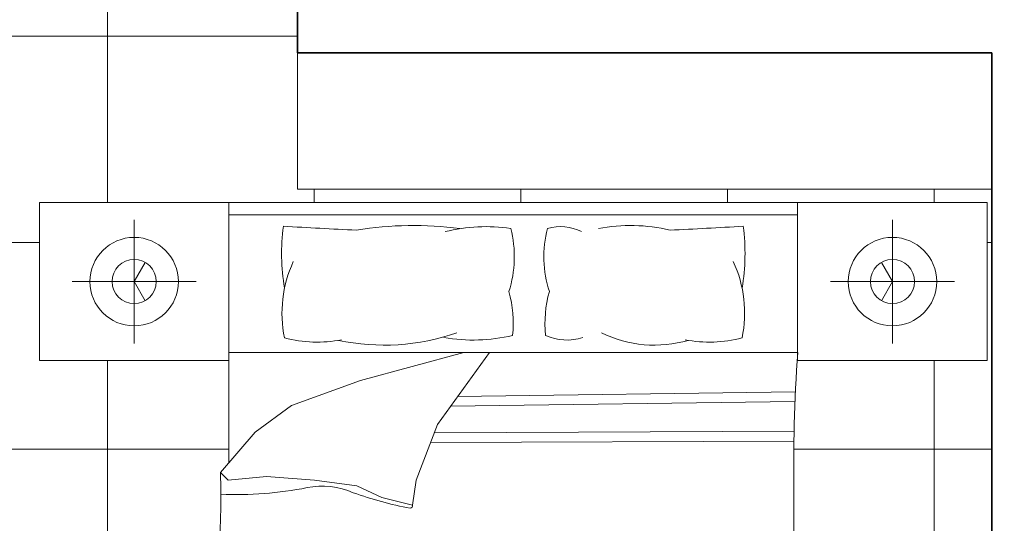
# Model space of a CAD drawing. Units: inches. Extents: x 351 to 1738, y -265 to 286.
# Tile 25 of 38: x 1127 to 1246, y 102 to 163. Entities that reach past the tile are written whole.
import ezdxf

# ---------------------------------------------------------------- set-up
doc = ezdxf.new("R2010")
doc.units = ezdxf.units.IN
doc.header["$MEASUREMENT"] = 0
for name, color, linetype, lineweight in [('A-FLOR-CASE', 9, 'Continuous', 18), ('A-FLOR-PATT', 9, 'Continuous', 9), ('A-FURN', 18, 'Continuous', 13), ('A-WALL', 7, 'Continuous', 35)]:
    doc.layers.add(name, color=color, linetype=linetype, lineweight=lineweight)

msp = doc.modelspace()

# ---------------------------------------------------------------- hatches: boundary and pattern name
at = {"layer": 'A-FLOR-PATT', "transparency": 33554559}
h = msp.add_hatch(dxfattribs=at)
h.set_pattern_fill('ANSI37', color=256, scale=200, angle=135)
h.set_pattern_definition([(180, (1112.704, -164.037), (-2e-15, -25), []), (270, (1112.704, -164.037), (25, -5e-15), [])])
h.paths.add_polyline_path([(1380.064, 73.463), (1380.132, 148.463), (1338.064, 148.463), (1290.704, 148.463), (1290.704, 88.463), (1248.704, 88.463), (1248.704, -2.009), (1244.704, -2.009), (1244.704, 142.457), (1160.704, 142.457), (1160.704, 158.963), (1160.704, 170.137), (1160.704, 206.137), (1160.704, 228.963), (1112.704, 228.963), (1112.704, 209.963), (1112.704, 168.963), (1124.704, 168.963), (1124.704, 162.963), (1112.704, 162.963), (1112.704, 64.463), (1112.704, 60.463), (1112.704, 0.463), (1112.704, -48.026), (1146.804, -47.981), (1146.804, -35.691), (1207.804, -35.691), (1207.804, -47.902), (1236.542, -47.864), (1236.544, -50.009), (1248.5, -50.009), (1248.506, -102.915), (1248.512, -150.915), (1248.514, -164.037), (1248.549, -164.037), (1273.017, -164.037), (1273.017, -128.799), (1355.24, -128.799), (1355.24, -164.037), (1384.204, -164.037), (1384.204, -57.037), (1380.064, -57.037), (1380.064, -48.037), (1392.064, -48.037), (1392.064, -53.037), (1406.549, -53.037), (1406.549, -57.037), (1401.204, -57.037), (1401.204, -147.037), (1468.204, -147.037), (1468.204, -138.5), (1472.204, -138.5), (1472.204, -102.5), (1468.204, -102.5), (1468.204, -57.037), (1442.549, -57.037), (1442.549, -53.037), (1463.049, -53.037), (1463.049, -40.747), (1524.049, -40.747), (1524.049, -48.037), (1536.064, -48.037), (1536.064, -53.037), (1557.704, -53.037), (1557.704, 204.963), (1384.204, 204.963), (1384.204, 73.463), (1392.064, 73.463), (1392.064, 64.463), (1384.204, 64.463), (1384.204, -3.5), (1380.204, -3.537), (1380.204, 64.463), (1380.064, 64.463)])
h.paths.add_polyline_path([(1510.714, 86.458, -0.1039845), (1511.661, 85.595, 0.4704384), (1510.158, 87.614, 0.0961001)], flags=16)
h.paths.add_polyline_path([(1510.443, 100.266, 0.009798), (1504.693, 100.48, 0.0287898), (1504.6, 99.767, -0.1653311), (1505.519, 96.135, -0.1436014)], flags=16)
h.paths.add_polyline_path([(1487.201, 85.595, -0.1039845), (1488.148, 86.458, 0.0961001), (1488.704, 87.614, 0.4704384)], flags=0)
h.paths.add_polyline_path([(1495.052, 100.43), (1494.178, 100.43, -0.0264629), (1494.262, 99.774, -0.1442193)], flags=16)
h.paths.add_polyline_path([(1444.485, 86.458, -0.1039845), (1445.433, 85.595, 0.4704384), (1443.93, 87.614, 0.0961001)], flags=16)
h.paths.add_polyline_path([(1420.972, 85.595, -0.1039845), (1421.92, 86.458, 0.0961001), (1422.475, 87.614, 0.4704384)], flags=16)
h.paths.add_polyline_path([(1428.632, 100.335, 0.0010541), (1427.971, 100.309, -0.0215241), (1428.033, 99.774, -0.1143008)], flags=16)
h.paths.add_polyline_path([(1419.906, 143.708, 0.0249793), (1420.222, 157.526), (1421.573, 159.101), (1421.573, 175.369), (1391.393, 175.369), (1391.393, 200.519), (1542.294, 200.519), (1542.294, 175.369), (1512.028, 175.369, 0.0198653), (1511.521, 153.838, 0.0251335), (1512.758, 118.323, 0.0205529), (1512.942, 115.253), (1419.834, 115.253, -0.0004142), (1419.843, 124.798), (1413.059, 124.798), (1413.059, 84.437, -0.0618528), (1415.831, 80.45, -0.0930773), (1420.972, 85.595, -0.2675367), (1422.371, 84.732, 0.0851103), (1424.052, 84.616, -0.8853927), (1424.033, 84.851, -1.1258145), (1424.073, 84.366, -0.0879871), (1422.371, 84.732, -0.2675367), (1422.326, 83.089, -0.3705421), (1420.972, 85.595, 0.0930773), (1415.831, 80.45, -0.0874142), (1417.914, 73.937), (1418.941, 73.937, 0.0272504), (1418.913, 76.906, -0.1157032), (1421.051, 73.937), (1445.354, 73.937, -0.1157032), (1447.492, 76.906, 0.0272504), (1447.464, 73.937), (1448.491, 73.937, -0.0874142), (1450.574, 80.45, 0.0930773), (1445.433, 85.595, -0.3705421), (1444.079, 83.089, -0.2675367), (1444.034, 84.732, -0.0879871), (1442.332, 84.366, -1.1258145), (1442.372, 84.851, -2.0327363), (1442.364, 84.368, 0.0863779), (1444.034, 84.732, -0.2675367), (1445.433, 85.595, -0.0930773), (1450.574, 80.45, -0.2577317), (1466.483, 90.927, -0.4786702), (1468.832, 91.907, -0.4786702), (1471.18, 90.927, -0.26264), (1483.053, 81.78, -0.0718662), (1487.201, 85.595, -0.2675367), (1488.6, 84.732, 0.0851103), (1490.28, 84.616, -0.8853927), (1490.262, 84.851, -1.1258145), (1490.301, 84.366, -0.0879871), (1488.6, 84.732, -0.2675367), (1488.554, 83.089, -0.3705421), (1487.201, 85.595, 0.0718662), (1483.053, 81.78, -0.1320648), (1484.143, 73.937), (1485.169, 73.937, 0.0272504), (1485.142, 76.906, -0.1157032), (1487.28, 73.937), (1511.582, 73.937, -0.1157032), (1513.72, 76.906, 0.0272504), (1513.693, 73.937), (1514.719, 73.937, -0.0874142), (1516.802, 80.45, 0.0930773), (1511.661, 85.595, -0.3705421), (1510.308, 83.089, -0.2675367), (1510.262, 84.732, -0.0879871), (1508.561, 84.366, -1.1258145), (1508.601, 84.851, -2.0327363), (1508.592, 84.368, 0.0863779), (1510.262, 84.732, -0.2675367), (1511.661, 85.595, -0.0930773), (1516.802, 80.45, -0.0618528), (1519.575, 84.437), (1519.575, 73.937), (1413.059, 73.937), (1413.059, 124.798), (1419.843, 124.798, -0.0008205)], flags=16)
h.paths.add_polyline_path([(1220.149, 54.133, -0.1039845), (1220.869, 53.476, 0.4704384), (1219.727, 55.011, 0.0961001)], flags=16)
h.paths.add_polyline_path([(1219.944, 64.626, 0.009798), (1215.574, 64.789, 0.0287898), (1215.503, 64.247, -0.1653311), (1216.201, 61.487, -0.1436014)], flags=16)
h.paths.add_polyline_path([(1209.779, 64.449, 0.0974459), (1209.339, 64.751), (1208.247, 64.751, 0.1273905), (1207.7, 64.326, 0.1715858), (1206.95, 61.475, -0.1588542), (1207.636, 59.45, 0.0158984), (1207.795, 59.218, 0.0615457), (1208.598, 59.616, 0.1754158), (1208.638, 60.099, -0.2847793), (1209.348, 62.472, 0.3262165)], flags=16)
h.paths.add_polyline_path([(1169.818, 54.133, -0.1039845), (1170.538, 53.476, 0.4704384), (1169.396, 55.011, 0.0961001)], flags=16)
h.paths.add_polyline_path([(1159.017, 62.472, 0.2847642), (1158.307, 60.099, -0.1754332), (1158.267, 59.616, 0.3929302), (1159.448, 64.449, -0.3262298)], flags=16)
h.paths.add_polyline_path([(1156.342, 58.239, -0.1783213), (1154.011, 55.31, -0.1747359), (1154.722, 55.233, -0.2008015), (1156.27, 56.086, 0.1269899), (1157.283, 58.991, -0.0912053)], flags=16)
h.paths.add_polyline_path([(1156.624, 61.413, 0.1572752), (1157.316, 64.247, 0.1696217)], flags=16)
h.paths.add_polyline_path([(1152.67, 54.133, -0.0961001), (1151.95, 53.476, 0.0640762), (1154.465, 54.384, 0.1990158)], flags=16)
h.paths.add_polyline_path([(1202.281, 53.476, -0.1039845), (1203, 54.133, 0.0961001), (1203.423, 55.011, 0.4704384)], flags=0)
h.paths.add_polyline_path([(1151.139, 97.64, 0.0249793), (1151.379, 108.141), (1152.406, 109.338), (1152.406, 121.701), (1129.47, 121.701), (1129.47, 140.814), (1244.149, 140.814), (1244.149, 121.701), (1221.148, 121.701, 0.0198653), (1220.763, 105.338, 0.0251335), (1221.703, 78.349, 0.0205529), (1221.843, 76.016), (1151.078, 76.016, -0.1287433), (1148.786, 65.037, 0.5393525), (1150.327, 64.171, -0.027594), (1163.481, 64.751, 0.0976954), (1163.04, 64.449, 0.3262165), (1163.471, 62.472, -0.2847765), (1164.181, 60.099, -0.1947567), (1165.846, 61.443, -0.1554021), (1165.172, 64.247, -0.1660224), (1165.869, 61.475, -0.1770142), (1167.852, 62.77, -0.4482027), (1169.974, 60.807, -0.3934987), (1167.679, 57.86, -0.8955483), (1168.438, 54.524, -0.3557668), (1166.218, 56.086, -0.066024), (1165.505, 57.539), (1165.251, 56.243, -0.3717324), (1164.02, 59.758, -0.3736141), (1163.04, 64.449, -0.0976954), (1163.481, 64.751, 0.0213538), (1153.294, 64.429, -0.1341826), (1156.695, 61.368, 0.1868727), (1154.636, 62.77, 0.4482027), (1152.514, 60.807, 0.4037263), (1154.905, 57.846, 0.7112192), (1153.334, 55, 0.5315397), (1151.95, 53.476, -0.2675367), (1153.013, 52.821, 0.0851103), (1154.29, 52.732, -0.8853927), (1154.276, 52.911, -1.1258145), (1154.306, 52.543, -0.0879871), (1153.013, 52.821, -0.2675367), (1152.978, 51.572, -0.3705421), (1151.95, 53.476, 0.0930773), (1148.043, 49.566, -0.0874142), (1149.626, 44.617), (1150.406, 44.617, 0.0272504), (1150.385, 46.873, -0.1157032), (1152.01, 44.617), (1170.478, 44.617, -0.1157032), (1172.103, 46.873, 0.0272504), (1172.082, 44.617), (1172.862, 44.617, -0.0874142), (1174.445, 49.566, 0.0930773), (1170.538, 53.476, -0.3705421), (1169.51, 51.572, -0.2675367), (1169.475, 52.821, -0.0879871), (1168.182, 52.543, -1.1258145), (1168.212, 52.911, -2.0327363), (1168.206, 52.544, 0.0863779), (1169.475, 52.821, -0.2675367), (1170.538, 53.476, -0.0930773), (1174.445, 49.566, -0.2577317), (1186.536, 57.528, -0.4786702), (1188.321, 58.273, -0.4786702), (1190.106, 57.528, -0.26264), (1199.128, 50.577, -0.0718662), (1202.281, 53.476, -0.2675367), (1203.344, 52.821, 0.0851103), (1204.621, 52.732, -0.8853927), (1204.607, 52.911, -1.1258145), (1204.637, 52.543, -0.0879871), (1203.344, 52.821, -0.2675367), (1203.309, 51.572, -0.3705421), (1202.281, 53.476, 0.0718662), (1199.128, 50.577, -0.1320648), (1199.957, 44.617), (1200.737, 44.617, 0.0272504), (1200.716, 46.873, -0.1157032), (1202.341, 44.617), (1220.809, 44.617, -0.1157032), (1222.434, 46.873, 0.0272504), (1222.413, 44.617), (1223.193, 44.617, -0.0874142), (1224.776, 49.566, 0.0930773), (1220.869, 53.476, -0.3705421), (1219.841, 51.572, -0.2675367), (1219.806, 52.821, -0.0879871), (1218.513, 52.543, -1.1258145), (1218.543, 52.911, -2.0327363), (1218.537, 52.544, 0.0863779), (1219.806, 52.821, -0.2675367), (1220.869, 53.476, -0.0930773), (1224.776, 49.566, -0.0618528), (1226.883, 52.597), (1226.883, 44.617), (1145.936, 44.617), (1145.936, 83.269), (1151.091, 83.269, -0.0008205)], flags=16)
h.paths.add_polyline_path([(1218.01, 57.86, -0.8955483), (1218.769, 54.524, -0.3557668), (1216.549, 56.086, -0.066024), (1215.836, 57.539), (1215.582, 56.243, -0.3717324), (1214.351, 59.758, -0.3736141), (1213.371, 64.449, 0.3262165), (1213.802, 62.472, -0.2847765), (1214.512, 60.099, -0.1947567), (1216.177, 61.443, -0.1799907), (1218.183, 62.77, -0.4482027), (1220.305, 60.807, -0.3934987)], flags=16)
h.paths.add_polyline_path([(1424.735, 91.363, -0.3934987), (1421.715, 95.241, -0.4482027), (1424.507, 97.824, -0.1799907), (1427.147, 96.077, -0.1947567), (1429.338, 94.309, -0.2847765), (1430.272, 97.432, 0.3262165), (1430.839, 100.034, -0.3736141), (1429.55, 93.861, -0.3717324), (1427.929, 89.235), (1427.596, 90.941, -0.066024), (1426.657, 89.029, -0.3557668), (1423.736, 86.973, -0.8955483)], flags=16)
h.paths.add_polyline_path([(1238.033, 131.257, -1), (1227.329, 131.257, -1)], flags=0)
h.paths.add_polyline_path([(1235.357, 131.257, -1), (1230.005, 131.257, -1)], flags=0)
h.paths.add_polyline_path([(1214.039, 54.243, 0.1543819), (1214.38, 53.992, 0.3589549), (1213.613, 54.016, 0.6039484), (1214.379, 53.657, 0.3713191), (1213.968, 52.872, 0.1879935), (1214.312, 52.809, -0.592455), (1213.953, 52.967, -0.2942791), (1214.083, 53.691, -1.3001871), (1213.881, 54.134, -0.2837621), (1214.469, 53.896, 1.1509396)], flags=16)
h.paths.add_polyline_path([(1212.091, 56.286, -0.4084338), (1211.337, 56.445, -0.0362594), (1211.098, 56.848, -0.2360976), (1211.59, 56.63, 0.0353445), (1211.835, 56.543, -0.4752408), (1212.091, 56.286, -0.4752408), (1212.438, 56.182, 0.0353445), (1212.631, 56.007, -0.2360976), (1213.056, 55.676, -0.0362594), (1212.588, 55.697, -0.4084338)], flags=16)
h.paths.add_polyline_path([(1211.469, 50.297, 0.296043), (1210.47, 50.527, 0.310883), (1211.931, 50.148, 0.0212546)], flags=16)
h.paths.add_polyline_path([(1213.739, 51.818, -0.0362594), (1213.271, 51.838, -0.4084337), (1212.774, 52.427, -0.0947856), (1212.293, 50.703, 1.1504738), (1212.911, 50.232, 0.1662877), (1213.265, 50.68, -0.0252543), (1212.603, 50.13, 1.0879317), (1212.471, 49.407, 0.1662877), (1213.02, 49.251, -0.016128), (1212.567, 49.563, -0.286859), (1212.217, 49.638, 0.0221563), (1212.046, 50.055, -0.6461302), (1212.185, 50.498, 0.0884116), (1212.732, 52.077, -1.1860374), (1213.121, 52.323, 0.0353445), (1213.314, 52.148, -0.2360976)], flags=16)
h.paths.add_polyline_path([(1212.094, 50.342, -0.0485241), (1211.54, 49.605, -1.1038339), (1211.397, 48.738, -0.7855147), (1211.683, 48.254, -0.3920429), (1210.948, 48.525, -0.3928194), (1210.561, 47.995, -0.592455), (1210.201, 48.153, -0.2942791), (1210.331, 48.877, -0.7041716), (1210.316, 49.592, -0.6793441), (1210.729, 50.112, 0.5636764)], flags=16)
h.paths.add_polyline_path([(1211.274, 49.829, -0.1398258), (1210.745, 49.859, -0.2178785), (1210.948, 49.509, -0.4985724)], flags=0)
h.paths.add_polyline_path([(1433.426, 81.49, -0.181571), (1434.245, 81.788, -0.0080665), (1433.726, 82.205, 0.0455784), (1432.755, 81.242, 0.1790113)], flags=16)
h.paths.add_polyline_path([(1434.146, 81.009, -0.1324418), (1433.645, 80.771, 0.2590893), (1433.234, 80.471, -0.1802109), (1433.392, 80.805, -0.1699398), (1432.758, 81.109, 0.0326525), (1433.273, 80.474, -0.4933627), (1434.046, 80.146, -0.3904966)], flags=16)
h.paths.add_polyline_path([(1434.83, 80.047, -0.9475376), (1435.294, 79.576, -0.2991282), (1434.625, 79.404, -0.2704392), (1435.01, 78.591, -0.592455), (1434.537, 78.382, -0.3928194), (1434.027, 79.08, -0.3920429), (1433.06, 78.723, -0.3520423), (1433.003, 79.197, -0.1972159), (1433.75, 79.734, -0.7136405), (1434.447, 79.939, -0.2147903), (1434.819, 80.475, 0.4088333), (1435.075, 80.803, -0.2261519)], flags=16)
h.paths.add_polyline_path([(1432.67, 81.217, -0.4542182), (1431.897, 79.923, -0.4144105), (1431.301, 80.035, 0.0161291), (1431.897, 80.445, 0.2795702), (1432.073, 80.871, -0.2895037), (1431.103, 81.321, -0.4144105), (1430.978, 81.915, 0.0161296), (1431.586, 81.521, 0.341293), (1432.125, 81.583, -0.8131856)], flags=16)
h.paths.add_polyline_path([(1429.893, 86.381, -0.9475376), (1430.358, 85.91, -0.1731062), (1429.984, 85.712, -0.0388172), (1431.625, 84.214, -0.0879005), (1432.097, 88.549, -0.0497684), (1431.254, 88.49, -0.2360976), (1431.814, 88.925, 0.0353445), (1432.067, 89.155, -0.4752408), (1432.524, 89.291, -0.4752408), (1432.86, 89.63, 0.0353445), (1433.182, 89.744, -0.2360976), (1433.83, 90.032, -0.0362594), (1433.516, 89.502, -0.4084338), (1432.524, 89.291, -0.3124239), (1432.106, 88.58, 0.0885594), (1431.625, 84.214, -0.4084337), (1430.971, 83.439, -0.0362594), (1430.355, 83.412, -0.2360976), (1430.914, 83.847, 0.0353445), (1431.168, 84.078, -0.4752408), (1431.625, 84.214, 0.0388172), (1429.984, 85.712, -0.3217316), (1429.333, 86.048, -0.32743), (1429.883, 86.809, 0.4088333), (1430.138, 87.138, -0.2261519)], flags=16)
h.paths.add_polyline_path([(1211.206, 58.616, -0.9997836), (1211.336, 59.323, -0.6149935)], flags=16)
h.paths.add_polyline_path([(1210.288, 49.429, 0.1543819), (1210.629, 49.178, 0.3589549), (1209.861, 49.202, 0.6039484), (1210.627, 48.843, -0.5348247), (1210.806, 49.295, 0.7483464)], flags=16)
h.paths.add_polyline_path([(1209.589, 51.828, -0.0087906), (1209.775, 51.753, 0.1122315), (1209.466, 52.019, 1.4188509), (1209.014, 51.708, -0.4587257), (1208.651, 51.073, -0.592455), (1208.291, 51.232, -0.2942791), (1208.421, 51.955, -1.3001871), (1208.219, 52.398, -0.2260052), (1208.719, 52.257, -0.4755189), (1209.158, 52.369, -1.4554994), (1209.603, 52.664, 0.4213049), (1209.191, 52.262, -0.5912116), (1208.979, 51.796, 0.4973986), (1209.773, 51.333, 0.6493116)], flags=16)
h.paths.add_polyline_path([(1208.029, 52.041, 0.5446671), (1208.832, 52.045, 0.220132)], flags=0)
h.paths.add_polyline_path([(1210.438, 51.425, -0.2041997), (1210.277, 52.018, 0.2708262), (1209.915, 52.897, 0.3241145)], flags=0)
h.paths.add_polyline_path([(1209.668, 52.407, -0.60139), (1208.99, 52.221, -0.3949159), (1208.248, 52.83, -0.8367916), (1208.651, 53.017, -0.3384876), (1209.039, 52.571, 0.1941379), (1209.191, 52.262, 0.4139945), (1209.712, 52.475, 0.5177103), (1210.503, 51.416, 0.401922), (1209.493, 50.93, 0.2063956), (1209.516, 50.165, -0.3194629), (1210.417, 51.418, -0.466635)], flags=16)
h.paths.add_polyline_path([(1206.601, 56.086, -0.3557668), (1204.381, 54.524, -0.9211983), (1205.236, 57.846, 0.2065693), (1207.614, 58.991, -0.1269899)], flags=16)
h.paths.add_polyline_path([(1435.487, 82.816, 0.5277653), (1436.615, 83.361, 0.5085402), (1437.05, 82.433, 0.592455), (1437.524, 82.641, 0.3312448), (1436.963, 83.548, 0.3878632), (1437.808, 83.626, 0.5929544), (1437.618, 84.176, 0.2260158), (1436.961, 83.99, 0.3182053), (1437.588, 84.854, 0.6893744), (1437.05, 84.991, 0.3357648), (1436.539, 84.41, -0.1569934), (1436.404, 84.065, -0.4346112), (1436.961, 83.99, -0.2147903), (1437.333, 84.526, 0.4088333), (1437.588, 84.854, -0.2261519), (1437.343, 84.097, -0.9475376), (1437.808, 83.626, -0.2991282), (1437.139, 83.455, -0.2704392), (1437.524, 82.641, -0.592455), (1437.05, 82.433, -0.3928194), (1436.541, 83.13, -0.4396601), (1435.475, 82.794, -0.174614), (1435.942, 82.244, -0.2063956), (1435.912, 81.237, -0.2708262), (1435.125, 82.208, 0.2079765), (1434.686, 82.904, -0.1964955)], flags=16)
h.paths.add_polyline_path([(1435.386, 84.832, 0.270811), (1434.91, 83.676, -0.2042174), (1434.699, 82.895, 0.3241145)], flags=0)
h.paths.add_polyline_path([(1435.68, 84.18, -0.2176564), (1435.554, 83.304, -0.1767045), (1436.236, 83.778, -0.3730364)], flags=0)
h.paths.add_polyline_path([(1435.566, 100.034, 0.3262165), (1436.133, 97.432, -0.2847765), (1437.067, 94.309, -0.1947567), (1439.258, 96.077, -0.1554021), (1438.371, 99.767, -0.1660224), (1439.289, 96.12, -0.1770142), (1441.897, 97.824, -0.4482027), (1444.69, 95.241, -0.3934987), (1441.67, 91.363, -0.8955483), (1442.669, 86.973, -0.3557668), (1439.748, 89.029, -0.066024), (1438.809, 90.941), (1438.476, 89.235, -0.3717324), (1436.855, 93.861, -0.3736141)], flags=16)
h.paths.add_polyline_path([(1191.252, 49.507, -0.2740221), (1190.658, 48.409, 0.2675367), (1191.311, 47.344, 0.3705421)], flags=0)
h.paths.add_polyline_path([(1190.301, 49.717, 0.1990158), (1188.619, 49.04, 0.0640762), (1191.252, 49.507, -0.0961001)], flags=0)
h.paths.add_polyline_path([(1189.518, 47.857, 1.1258145), (1189.676, 47.523, 2.0446052)], flags=0)
h.paths.add_polyline_path([(1464.974, 80.372, 0.2740221), (1465.756, 78.927, -0.0830131)], flags=0)
h.paths.add_polyline_path([(1464.974, 80.372, 0.3705421), (1464.897, 77.525, 0.5763244)], flags=0)
h.paths.add_polyline_path([(1464.974, 80.372, -0.4704384), (1467.284, 81.372, -0.0961001), (1466.226, 80.648, -0.1990158), (1468.439, 79.757, -0.0640762)], flags=0)
h.paths.add_polyline_path([(1189.511, 56.43, -0.2594668), (1188.321, 56.391, -0.2594668), (1187.13, 56.43, 0.0851103), (1188.193, 55.716, -0.8853927), (1188.27, 55.878, -1.1960133), (1188.355, 55.442, 0.1014587)], flags=0)
h.paths.add_polyline_path([(1188.321, 57.596, 0.0780722), (1187.678, 57.24, 0.0155503), (1188.321, 57.136, 0.0155503), (1188.964, 57.24, 0.0780722)], flags=0)
h.paths.add_polyline_path([(1190.164, 55.365, -0.5763244), (1190.106, 57.528, -0.1982945), (1188.321, 58.319, -0.1982945), (1186.536, 57.528, -0.5763244), (1186.477, 55.365, -0.3705421), (1186.536, 57.528, 0.1982945), (1188.321, 58.319, 0.1982945), (1190.106, 57.528, -0.3705421)], flags=0)
h.paths.add_polyline_path([(1188.372, 55.878, 1.1258145), (1188.529, 55.544, 2.0446052)], flags=0)
h.paths.add_polyline_path([(1186.341, 49.717, -0.0961001), (1185.389, 49.507, 0.0640762), (1188.022, 49.04, 0.1990158)], flags=0)
h.paths.add_polyline_path([(1185.389, 49.507, -0.2675367), (1185.984, 48.409, 0.0851103), (1187.046, 47.695, -0.8853927), (1187.123, 47.857, -1.1258145), (1186.966, 47.523, -0.0879871), (1185.984, 48.409, -0.2675367), (1185.331, 47.344, -0.3705421)], flags=0)
h.paths.add_polyline_path([(1399.441, 187.944, -1), (1413.525, 187.944, -1)], flags=0)
h.paths.add_polyline_path([(1402.962, 187.944, -1), (1410.004, 187.944, -1)], flags=0)
h.paths.add_polyline_path([(1357.663, -72.245), (1377.272, -72.245), (1377.272, -91.854), (1357.663, -91.854)], flags=16)
h.paths.add_polyline_path([(1467.256, 78.201, -1.1258145), (1467.049, 77.761, -2.0446052)], flags=0)
h.paths.add_polyline_path([(1468.822, 88.714, 0.9411249), (1469.106, 88.316, 1.1371523), (1468.765, 88.755, 0.890986), (1468.99, 88.245, 0.0948283), (1470.398, 89.481, -0.2675367), (1471.18, 90.927, -0.0281232), (1469.678, 90.547, -0.0287737), (1469.948, 90.311, -0.0203267), (1468.832, 90.41, -0.0203267), (1467.716, 90.311, -0.0287737), (1467.986, 90.547, -0.0281232), (1466.483, 90.927, -0.2675367), (1467.265, 89.481, 0.0851103), (1468.663, 88.542, -1.2023159)], flags=0)
h.paths.add_polyline_path([(1178.25, 124.523, -0.1199286), (1165.65, 124.145, -0.1073492), (1159.133, 124.446, -0.1028906), (1159.132, 130.465, -0.0748968), (1158.993, 137.956, 0.002027), (1167.844, 137.479, -0.07553), (1180.337, 137.666, -0.0758613), (1186.502, 137.688, -0.1409896), (1186.272, 130.046, -0.0954805), (1186.729, 124.748, -0.10603)], flags=0)
h.paths.add_polyline_path([(1469.225, 79.757, -0.1990158), (1471.437, 80.648, -0.0961001), (1470.379, 81.372, -0.4704384), (1472.689, 80.372, -0.3705421), (1472.766, 77.525, -0.2675367), (1471.907, 78.927, -0.0879863), (1470.615, 77.761, -1.1258491), (1470.408, 78.201, -2.0327363), (1470.642, 77.778, 0.0863779), (1471.907, 78.927, -0.2675367), (1472.689, 80.372, -0.0640762)], flags=0)
h.paths.add_polyline_path([(1430.423, 186.902, -0.0748968), (1430.24, 196.758, 0.002027), (1441.887, 196.131, -0.07553), (1458.326, 196.377, -0.0758613), (1466.438, 196.406, -0.1409896), (1466.136, 186.35, -0.0954805), (1466.737, 179.378, -0.10603), (1455.58, 179.082, -0.1199286), (1439, 178.585, -0.1073492), (1430.425, 178.981, -0.1028906)], flags=0)
h.paths.add_polyline_path([(1162.258, 49.939, 0.3357645), (1161.87, 49.497, -0.1569936), (1161.767, 49.235, -0.4346112), (1162.19, 49.178, -0.2147903), (1162.473, 49.585, 1.5291948)], flags=16)
h.paths.add_polyline_path([(1161.683, 49.021, 0.5815181), (1161.268, 49.583, 0.5927609)], flags=16)
h.paths.add_polyline_path([(1162.602, 48.058, 0.3713191), (1162.192, 48.843, 0.4345332), (1162.88, 48.962, 0.1850806), (1162.197, 48.926, 1.1218369)], flags=16)
h.paths.add_polyline_path([(1161.443, 48.941, -1.3071038), (1161.495, 48.571, -0.2177521), (1161.136, 48.254, 0.6973029), (1161.871, 49.048, 0.1215141)], flags=16)
h.paths.add_polyline_path([(1162.531, 49.429, -0.2070837), (1162.05, 49.146, -0.9920299)], flags=16)
h.paths.add_polyline_path([(1161.304, 49.578, -0.7196675), (1161.513, 50.079, -0.1304275), (1160.836, 50.168, 0.0395926)], flags=0)
h.paths.add_polyline_path([(1162.036, 50.584, -0.0080665), (1161.642, 50.9, 0.0293675), (1161.35, 50.297, -0.2057884)], flags=16)
h.paths.add_polyline_path([(1162.882, 51.392, -0.1247327), (1162.763, 51.828, -0.1011907), (1162.399, 51.438, -0.153425)], flags=0)
h.paths.add_polyline_path([(1164.235, 51.85, -0.3091075), (1164.513, 51.136, -0.6271245), (1163.781, 51.603, -0.6859091), (1162.777, 51.219, -0.2332851), (1163.303, 50.165, -0.2708262), (1162.705, 50.903, 0.2041997), (1162.381, 51.425, 0.204182), (1162.542, 52.018, -0.2708414), (1162.903, 52.897, -0.1272607), (1163.219, 52.529, -1.1686811), (1163.781, 52.587, -0.3291117), (1164.168, 53.017, -0.8367917), (1164.571, 52.83, -0.1933406), (1164.391, 52.338, -0.9475376), (1164.744, 51.981, -0.2991282)], flags=16)
h.paths.add_polyline_path([(1163.598, 51.937, -1.2629561), (1163.236, 51.831, 0.0125754), (1162.971, 51.721, 0.2306566), (1163.151, 52.407, -0.1648982), (1163.178, 52.661, -0.4493201), (1163.628, 52.262, -0.721477), (1164.154, 52.088, -0.8499982)], flags=0)
h.paths.add_polyline_path([(1161.613, 58.616, -0.9804131), (1161.525, 59.049, -2.9089348)], flags=16)
h.paths.add_polyline_path([(1160.252, 49.166, -0.4144105), (1159.799, 49.251, 0.0161291), (1160.252, 49.563, 0.2795702), (1160.386, 49.887, -0.2895037), (1159.649, 50.229, -0.4144105), (1159.554, 50.68, 0.0161296), (1160.015, 50.381, 0.6178854), (1160.526, 50.703, -0.0947856), (1160.045, 52.427, -0.1404436), (1159.682, 52.042, -0.0578559), (1159.3, 51.872, 0.5448433), (1160.046, 52.419, -0.0881216), (1160.404, 55.721, -0.0497684), (1159.763, 55.676, -0.2360976), (1160.188, 56.007, 0.0353445), (1160.381, 56.182, -0.4752408), (1160.728, 56.286, -0.4752408), (1160.984, 56.543, 0.0353445), (1161.229, 56.63, -0.2360976), (1161.721, 56.848, -0.0362594), (1161.482, 56.445, -0.4084338), (1160.728, 56.286, -0.3124239), (1160.411, 55.745, 0.0885594), (1160.045, 52.427, 0.1070813), (1160.634, 50.498, -0.4947977), (1160.839, 50.149, -0.4542182)], flags=16)
h.paths.add_polyline_path([(1160.666, 49.808, -2.0765276), (1160.828, 50.172, 0.0195861)], flags=0)
h.paths.add_polyline_path([(1158.439, 53.992, 0.1543819), (1158.78, 54.243, 0.7483463), (1158.262, 54.109, -0.3382251), (1158.492, 53.839, -0.1708158), (1159.124, 53.779, 0.4957286), (1158.938, 54.134, 0.2260157)], flags=16)
h.paths.add_polyline_path([(1160.045, 52.427, 0.0388172), (1158.798, 53.565, -0.1198178), (1158.574, 53.586, -0.3091075), (1158.851, 52.872, -0.1879935), (1158.506, 52.809, 0.592455), (1158.866, 52.967, 0.3312448), (1158.44, 53.657, 0.2012451), (1158.798, 53.565, -0.034023), (1159.901, 52.578, -0.0442527), (1159.698, 52.323, -0.4752408)], flags=16)
h.paths.add_polyline_path([(1336.926, -95.392), (1336.926, -117.945), (1291.82, -117.945), (1291.82, -95.392)], flags=16)
h.paths.add_polyline_path([(1357.535, -97.244), (1357.726, -96.697, 0.0348443)], flags=16)
h.paths.add_polyline_path([(1376.693, -96.478), (1377.301, -96.5, 0.0314968), (1375.907, -96.424), (1357.726, -96.424)], flags=16)
h.paths.add_polyline_path([(1379.403, -119.667, 0.0267056), (1380.043, -119.439, -0.0152991)], flags=16)
h.paths.add_polyline_path([(1357.726, -120.202), (1357.821, -120.202), (1357.821, -120.201)], flags=16)
h.paths.add_polyline_path([(1354.171, -104.592), (1354.469, -98.672, 0.0111377)], flags=16)
h.paths.add_polyline_path([(1355.058, -119.136), (1354.578, -118.539, 0.1431635)], flags=16)
h.paths.add_polyline_path([(1378.851, -96.821), (1378.85, -96.82), (1378.85, -96.82, -0.0496798), (1380.055, -97.191), (1378.85, -96.82, 0.1500541), (1375.135, -97.188), (1375.136, -119.44, -0.0099698), (1374.747, -116.649), (1357.726, -116.649, 0.1693849), (1357.535, -119.382), (1357.535, -119.382), (1357.535, -119.382, 0.0348176), (1357.726, -119.928), (1357.726, -119.928), (1357.726, -119.929, -0.0348772), (1357.535, -119.382), (1355.507, -119.382), (1355.317, -119.278), (1357.535, -119.382, -0.1693939), (1357.726, -116.649, -0.0391513), (1374.686, -116.113, -0.0020149), (1374.625, -115.546, 0.1153223), (1369.915, -115.474, 0.0609215), (1369.922, -101.154, 0.1151459), (1374.625, -101.079, -0.0020164), (1374.686, -100.513, -0.0391511), (1357.726, -99.977), (1374.747, -99.977, -0.0099633), (1375.135, -97.188), (1375.135, -97.188, -0.1501081)], flags=16)
h.paths.add_polyline_path([(1490.963, 91.363, -0.3934987), (1487.944, 95.241, -0.4482027), (1490.736, 97.824, -0.1799907), (1493.376, 96.077, -0.1947567), (1495.567, 94.309, -0.2847765), (1496.501, 97.432, 0.3262165), (1497.068, 100.034, -0.3736141), (1495.778, 93.861, -0.3717324), (1494.158, 89.235), (1493.824, 90.941, -0.066024), (1492.886, 89.029, -0.3557668), (1489.964, 86.973, -0.8955483)], flags=16)
h.paths.add_polyline_path([(1354.86, -97.658), (1355.316, -97.348, 0.1019112)], flags=16)
h.paths.add_polyline_path([(1497.063, 83.327, 0.1767244), (1496.37, 83.785, -0.4051388), (1496.016, 83.384, 0.4973986), (1497.06, 82.774, 0.6493116), (1496.818, 83.426, -0.0087906)], flags=16)
h.paths.add_polyline_path([(1496.339, 83.783, 0.5927609), (1496.886, 84.522, 0.5815181)], flags=16)
h.paths.add_polyline_path([(1495.11, 82.641, 0.592455), (1495.583, 82.433, 0.6769152), (1495.805, 83.59, 0.3756693)], flags=16)
h.paths.add_polyline_path([(1495.015, 84.176, -0.145057), (1495.301, 84.526, -0.4088333), (1495.045, 84.854, 0.2206292), (1495.381, 84.152, -0.199594), (1495.851, 83.764, -0.5240172), (1494.826, 83.626, -0.5929976)], flags=16)
h.paths.add_polyline_path([(1501.655, 81.915, -0.0161291), (1501.048, 81.521, -0.3927187), (1500.462, 81.37, -0.2106699), (1500.607, 81.142, 0.3066994)], flags=16)
h.paths.add_polyline_path([(1500.11, 89.291, -0.4084338), (1499.118, 89.502, -0.0362594), (1498.803, 90.032, -0.2360976), (1499.451, 89.744, 0.0353445), (1499.774, 89.63, -0.4752408), (1500.11, 89.291, -0.4752408), (1500.567, 89.155, 0.0353445), (1500.82, 88.925, -0.2360976), (1501.379, 88.49, -0.0362594), (1500.763, 88.516, -0.4084338)], flags=16)
h.paths.add_polyline_path([(1498.908, 82.205, -0.0513217), (1500.013, 81.134, -0.5879306), (1500.234, 81.676, 0.1070813), (1501.009, 84.214, -0.03529)], flags=16)
h.paths.add_polyline_path([(1496.93, 83.875, -0.2063956), (1497.247, 84.832, -0.2708262), (1497.724, 83.676, 0.2079765), (1497.944, 82.884, -0.3814554)], flags=16)
h.paths.add_polyline_path([(1496.721, 81.237, 0.2708125), (1497.509, 82.208, -0.2042157), (1497.935, 82.895, 0.3241145)], flags=16)
h.paths.add_polyline_path([(1497.529, 80.125, -0.145057), (1497.814, 80.475, -0.703182), (1498.282, 81.178, -0.1229248), (1497.977, 81.714, -0.2708368), (1499.207, 81.49, 0.2079641), (1499.993, 81.248, -0.2651454), (1499.278, 80.472, 0.3819006), (1498.808, 79.947, -0.3059049), (1498.848, 79.519, 0.4994816), (1498.574, 79.217, -0.4587257), (1498.097, 78.382, -0.592455), (1497.624, 78.591, -0.2704392), (1498.009, 79.404, -0.299116), (1497.34, 79.576, -0.5930157)], flags=16)
h.paths.add_polyline_path([(1500.736, 79.923, 0.4144105), (1501.333, 80.035, -0.3216484), (1500.192, 80.765, 0.0198856), (1499.976, 81.251, 0.4653307)], flags=16)
h.paths.add_polyline_path([(1501.009, 84.214, -0.0388172), (1502.649, 85.712, -0.1730946), (1502.276, 85.91, -0.5930157), (1502.465, 86.46, -0.145057), (1502.751, 86.809, -0.4088333), (1502.495, 87.138, 0.2206292), (1502.831, 86.436, -0.199594), (1503.301, 86.048, -0.3217316), (1502.649, 85.712, 0.0388172), (1501.009, 84.214, 0.1224486), (1501.412, 83.755, 0.4754908), (1501.335, 84.226, 0.055822), (1501.719, 83.847, -0.2360976), (1502.278, 83.412, -0.0362594), (1501.663, 83.439, -0.4084338)], flags=16)
h.paths.add_polyline_path([(1501.794, 100.034, 0.3262165), (1502.362, 97.432, -0.2847765), (1503.295, 94.309, -0.1947567), (1505.486, 96.077, -0.1799907), (1508.126, 97.824, -0.4482027), (1510.918, 95.241, -0.3934987), (1507.899, 91.363, -0.8955483), (1508.898, 86.973, -0.3557668), (1505.976, 89.029, -0.066024), (1505.038, 90.941), (1504.704, 89.235, -0.3717324), (1503.084, 93.861, -0.3736141)], flags=16)
h.paths.add_polyline_path([(1146.29, 131.257, -1), (1135.587, 131.257, -1)], flags=0)
h.paths.add_polyline_path([(1143.614, 131.257, -1), (1138.262, 131.257, -1)], flags=0)
h.paths.add_polyline_path([(1524.064, 73.463), (1536.064, 73.463), (1536.064, 64.463), (1524.064, 64.463)], flags=16)
h.paths.add_polyline_path([(1520.162, 187.944, -1), (1534.246, 187.944, -1)], flags=0)
h.paths.add_polyline_path([(1530.725, 187.944), (1527.204, 187.944), (1527.204, 184.423, 0.4142136)], flags=0)
h.paths.add_polyline_path([(1278.415, -91.154), (1331.067, -91.154), (1331.067, -80.583), (1278.415, -80.583)], flags=24)
h.paths.add_polyline_path([(1266.655, -79.354), (1354.738, -79.354), (1354.738, -67.817), (1266.655, -67.817)], flags=24)
h.paths.add_polyline_path([(1115.482, 206.184), (1155.098, 206.184), (1155.098, 217.714), (1115.482, 217.714)], flags=24)
h.paths.add_polyline_path([(1161.771, 8.501), (1222.466, 8.501), (1222.466, 19.079), (1161.771, 19.079)], flags=24)
h.paths.add_polyline_path([(1164.656, 18.795), (1210.615, 18.795), (1210.615, 30.324), (1164.656, 30.324)], flags=24)
h.paths.add_polyline_path([(1368.147, -32.882), (1379.362, -32.882), (1379.362, -21.733), (1368.147, -21.733)], flags=24)
h.paths.add_polyline_path([(1244.842, -31.012), (1256.057, -31.012), (1256.057, -19.863), (1244.842, -19.863)], flags=24)
h.paths.add_polyline_path([(1114.589, 195.739), (1156.517, 195.739), (1156.517, 206.31), (1114.589, 206.31)], flags=24)
h.paths.add_polyline_path([(1436.398, 37.632), (1505.131, 37.632), (1505.131, 48.203), (1436.398, 48.203)], flags=24)
h.paths.add_polyline_path([(1435.991, 47.919), (1507.906, 47.919), (1507.906, 59.456), (1435.991, 59.456)], flags=24)
h.paths.add_polyline_path([(1415.107, -124.896), (1457.038, -124.896), (1457.038, -114.318), (1415.107, -114.318)], flags=24)
h.paths.add_polyline_path([(1417.992, -114.602), (1457.609, -114.602), (1457.609, -103.073), (1417.992, -103.073)], flags=24)

# ---------------------------------------------------------------- linework, layer by layer
at = {"layer": 'A-FLOR-CASE'}
for p, q in [((1160.704, 158.963), (1160.704, 142.457)), ((1160.704, 142.457), (1244.704, 142.457))]:
    msp.add_line(p, q, dxfattribs=at)
at = {"layer": 'A-FURN'}
for p, q in [((1152.406, 140.814), (1152.406, 109.338)), ((1140.938, 123.765), (1140.938, 138.75)), ((1221.213, 139.342), (1152.406, 139.342)), ((1232.681, 123.765), (1232.681, 138.75)), ((1148.431, 131.257), (1133.446, 131.257)), ((1225.189, 131.257), (1240.173, 131.257)), ((1152.406, 122.691), (1221.213, 122.691)), ((1220.861, 116.75), (1179.22, 116.162)), ((1220.905, 117.927), (1180.077, 117.355)), ((1220.802, 113.14), (1177.255, 112.967)), ((1220.807, 111.962), (1176.806, 111.782))]:
    msp.add_line(p, q, dxfattribs=at)
for points in [[(1152.406, 121.701), (1129.47, 121.701), (1129.47, 140.814), (1244.149, 140.814), (1244.149, 121.701), (1221.213, 121.701), (1221.213, 140.814)], [(1142.276, 128.94), (1140.938, 131.257), (1142.276, 133.575)], [(1231.343, 133.575), (1232.681, 131.257), (1231.343, 128.94)], [(1183.91, 122.691), (1177.626, 113.944), (1175.071, 107.212), (1174.607, 104.195), (1170.89, 105.123), (1167.871, 106.516), (1162.761, 107.212), (1156.954, 107.677), (1152.309, 107.212), (1151.379, 108.141), (1155.56, 113.016), (1159.973, 116.265), (1168.335, 119.283), (1180.84, 122.691)]]:
    msp.add_lwpolyline(points, dxfattribs=at)
for points in [[(1158.993, 137.956, 0.0748968), (1159.132, 130.465, -0.4728166)], [(1186.272, 130.046, 0.1409896), (1186.502, 137.688, 0.2352448)], [(1191.169, 130.046, -0.1409896), (1190.94, 137.688, -0.2352448)], [(1214.626, 137.956, -0.0748968), (1214.487, 130.465, 0.4728166)]]:
    msp.add_lwpolyline(points, format="xyb", dxfattribs=at)
for centre, radius in [((1140.938, 131.257), 5.352), ((1232.681, 131.257), 5.352), ((1140.938, 131.257), 2.676), ((1232.681, 131.257), 2.676)]:
    msp.add_circle(centre, radius, dxfattribs=at)
for centre, radius, start, end in [((1222.203, 1229.315), 1093.188, 266.685209, 267.149775), ((1174.706, 96.458), 41.591, 82.21958, 99.49698), ((1183.49, 117.477), 20.434, 81.52493, 103.95996), ((1192.514, 132.237), 5.673, 63.34374, 106.10256), ((1201.015, 117.89), 20.16, 76.34271, 101.1841), ((1151.416, 1229.315), 1093.188, 272.850225, 273.314791), ((1173.603, 127.458), 14.78, 155.1316, 191.75834), ((1200.016, 127.458), 14.78, 348.24166, 24.8684), ((1172.754, 126.214), 14.051, 354.01289, 15.82928), ((1204.688, 126.214), 14.051, 164.17072, 185.98711), ((1163.084, 139.298), 15.368, 255.10393, 281.03689), ((1171.174, 150.222), 26.655, 258.03974, 289.26152), ((1181.965, 144.402), 20.223, 259.86169, 283.62376), ((1193.281, 130.259), 6.079, 245.01826, 288.54073), ((1203.903, 138.166), 14.598, 243.87611, 286.17464), ((1210.536, 139.298), 15.368, 258.96311, 284.89607), ((1426.794, 108.676), 206.058, 176.09997, 180.92818), ((1046.231, 105.29), 105.187, 355.82941, 1.55305), ((1153.342, 148.751), 43.281, 267.45188, 281.3392), ((1163.687, 97.162), 9.335, 66.26158, 101.3392), ((1182.569, 147.53), 44.473, 250.11942, 259.33829), ((1489.524, 101.184), 268.793, 179.11454, 184.87351), ((1174.346, 104.101), 0.277, 268.86235, 19.75363)]:
    msp.add_arc(centre, radius, start, end, dxfattribs=at)
at = {"layer": 'A-WALL'}
for p, q in [((1160.704, 158.963), (1160.704, 170.137)), ((1160.704, 158.963), (1244.704, 158.963)), ((1244.704, -2.009), (1244.704, 158.963))]:
    msp.add_line(p, q, dxfattribs=at)

doc.saveas('drawing.dxf')
